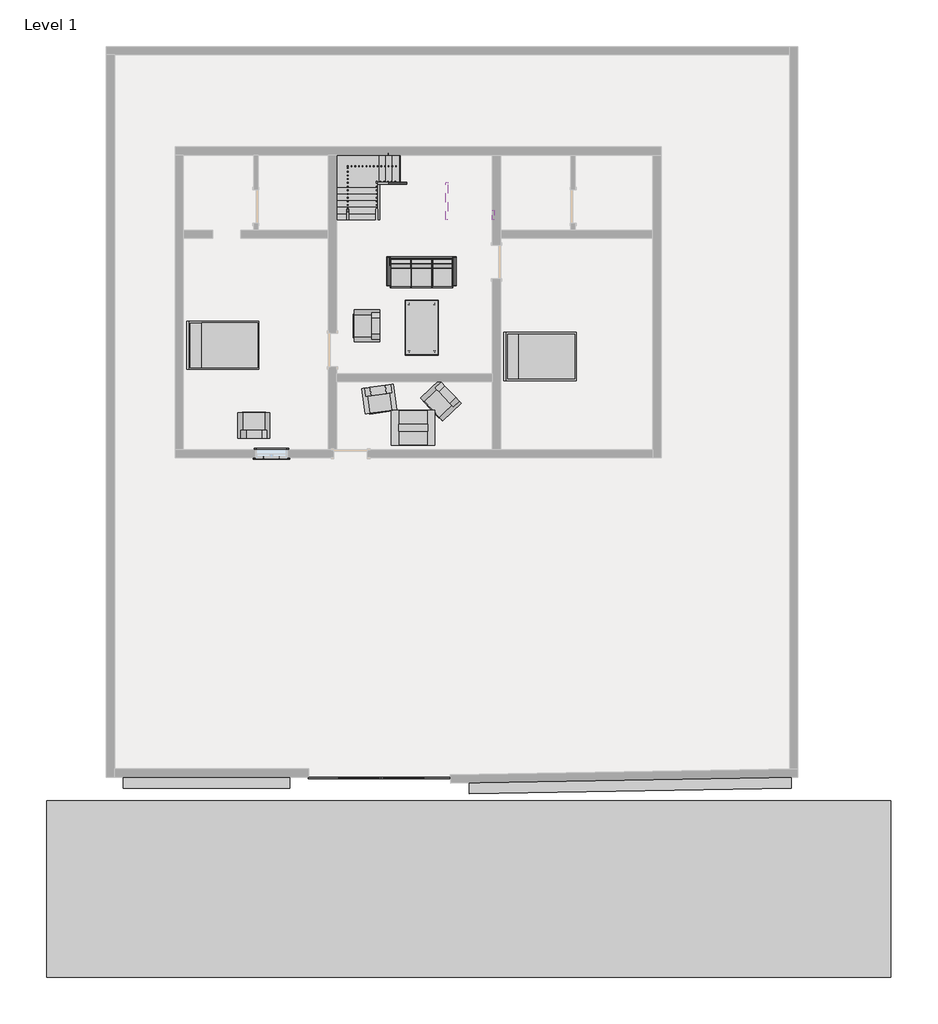
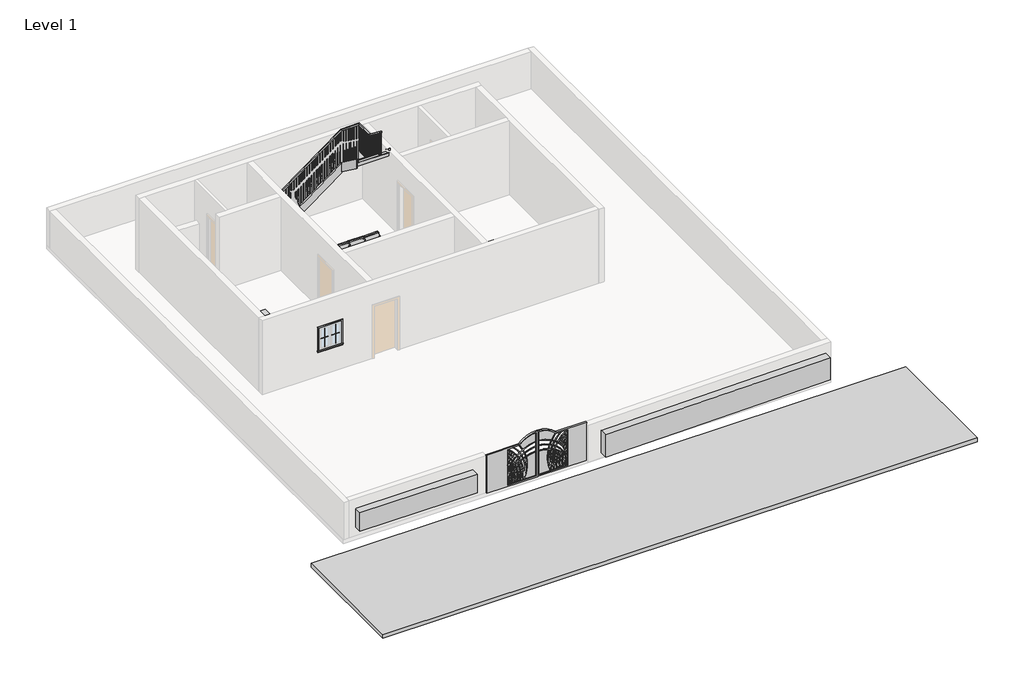
# One storey, part 2 of 2: 9 furniture elements, 8 proxies, 6 members, 1 railing, 1 stair flight.
"""IFC4 building model written with IfcOpenShell, lengths in millimetres."""

from ifc_helpers import new_model, si_unit, frame, origin, place, context, project, spatial, polyline, outline, extrude, faceted_brep, transform, mapped, element, save
from components import generic_models_1_generic_models_1_de819adb, generic_models_2_generic_models_2_5d5211df, generic_models_3_generic_models_3_fb8d8730, muntin_pattern_2x2_muntin_pattern_2x2_b3fe6957, muntin_pattern_2x2_muntin_pattern_2x2_3e0ecaf2, trim_window_exterior_flat_with_sill_41619996, trim_window_interior_flat_picture_frame_51c85655, gate_7956_gate_7956_2a423054, furniture_2fc85b74, furniture_29a9adb8, furniture_57072a26, bed_17739_bed_17739_15c61121, chair_lounge_11461_couch_0866092f, dining_table_14755_dining_table_14755_d89cb775, wood_and_glass_coffee_table_17065_wood_and_glass_coffee_dbc724b2, stair_flight_92e1e4df

model = new_model("IFC4")

# Units and contexts
model_context = context("Model", 3, world=origin())
ifc_project = project(units=[si_unit("LENGTHUNIT", "METRE", prefix="MILLI")], contexts=[model_context])

# Site, building, storey
site = spatial("IfcSite", under=ifc_project)
building = spatial("IfcBuilding", under=site)
storey = spatial("IfcBuildingStorey", under=building, Name="Level 1", Elevation=0.0)

# Proxies
placement = place(None, origin())
generic_models_1_generic_models_1_shape = generic_models_1_generic_models_1_de819adb(model_context)
element("IfcBuildingElementProxy", 1, Name="Generic Models 1 : Generic Models 1", ObjectType="Generic Models 1 : Generic Models 1", at=placement, inside=storey, context=model_context, shape_type="MappedRepresentation", body=[
    mapped(generic_models_1_generic_models_1_shape, transform((0.0, 0.0, 0.0), x_axis=(1.0, 0.0, 0.0), y_axis=(0.0, 1.0, 0.0), z_axis=(0.0, 0.0, 1.0))),
])
generic_models_2_generic_models_2_shape = generic_models_2_generic_models_2_5d5211df(model_context)
element("IfcBuildingElementProxy", 2, Name="Generic Models 2 : Generic Models 2", ObjectType="Generic Models 2 : Generic Models 2", at=placement, inside=storey, context=model_context, shape_type="MappedRepresentation", body=[
    mapped(generic_models_2_generic_models_2_shape, transform((0.0, 0.0, 0.0), x_axis=(1.0, 0.0, 0.0), y_axis=(0.0, 1.0, 0.0), z_axis=(0.0, 0.0, 1.0))),
])
generic_models_3_generic_models_3_shape = generic_models_3_generic_models_3_fb8d8730(model_context)
element("IfcBuildingElementProxy", 3, Name="Generic Models 3 : Generic Models 3", ObjectType="Generic Models 3 : Generic Models 3", at=placement, inside=storey, context=model_context, shape_type="MappedRepresentation", body=[
    mapped(generic_models_3_generic_models_3_shape, transform((0.0, 0.0, 0.0), x_axis=(1.0, 0.0, 0.0), y_axis=(0.0, 1.0, 0.0), z_axis=(0.0, 0.0, 1.0))),
])
muntin_pattern_2x2_muntin_pattern_2x2_shape = muntin_pattern_2x2_muntin_pattern_2x2_b3fe6957(model_context)
element("IfcBuildingElementProxy", 4, Name="Muntin Pattern_2x2 : Muntin Pattern_2x2", ObjectType="Muntin Pattern_2x2 : Muntin Pattern_2x2", at=placement, inside=storey, context=model_context, shape_type="MappedRepresentation", body=[
    mapped(muntin_pattern_2x2_muntin_pattern_2x2_shape, transform((-5069.3921642, -1799.3582394, 1136.9934313), x_axis=(-1.0, 0.0, 0.0), y_axis=(0.0, -1.0, 0.0), z_axis=(0.0, 0.0, 1.0))),
])
muntin_pattern_2x2_muntin_pattern_2x2_2_shape = muntin_pattern_2x2_muntin_pattern_2x2_3e0ecaf2(model_context)
element("IfcBuildingElementProxy", 5, Name="Muntin Pattern_2x2 : Muntin Pattern_2x2", ObjectType="Muntin Pattern_2x2 : Muntin Pattern_2x2", at=placement, inside=storey, context=model_context, shape_type="MappedRepresentation", body=[
    mapped(muntin_pattern_2x2_muntin_pattern_2x2_2_shape, transform((-5498.0171642, -1799.3582394, 1136.9934313), x_axis=(1.0, 0.0, 0.0), y_axis=(0.0, 1.0, 0.0), z_axis=(0.0, 0.0, 1.0))),
])
trim_window_exterior_flat_with_sill_shape = trim_window_exterior_flat_with_sill_41619996(model_context)
element("IfcBuildingElementProxy", 6, Name="Trim-Window-Exterior-Flat : with Sill", ObjectType="Trim-Window-Exterior-Flat : with Sill", at=placement, inside=storey, context=model_context, shape_type="MappedRepresentation", body=[
    mapped(trim_window_exterior_flat_with_sill_shape, transform((-5283.7046642, -1808.8832394, 1981.5434313), x_axis=(1.0, 0.0, 0.0), y_axis=(0.0, 0.0, 1.0), z_axis=(0.0, -1.0, 0.0))),
])
trim_window_interior_flat_picture_frame_shape = trim_window_interior_flat_picture_frame_51c85655(model_context)
element("IfcBuildingElementProxy", 7, Name="Trim-Window-Interior-Flat : Picture Frame", ObjectType="Trim-Window-Interior-Flat : Picture Frame", at=placement, inside=storey, context=model_context, shape_type="MappedRepresentation", body=[
    mapped(trim_window_interior_flat_picture_frame_shape, transform((-5283.7046642, -1580.2832394, 1981.5434313), x_axis=(-1.0, 0.0, 0.0), y_axis=(0.0, 0.0, 1.0), z_axis=(0.0, 1.0, 0.0))),
])
gate_7956_gate_7956_shape = gate_7956_gate_7956_2a423054(model_context)
element("IfcBuildingElementProxy", 8, Name="gate_7956 : gate_7956", ObjectType="gate_7956 : gate_7956", at=placement, inside=storey, context=model_context, shape_type="MappedRepresentation", body=[
    mapped(gate_7956_gate_7956_shape, transform((-2281.8126986, -10566.5980165, 0.0), x_axis=(1.0, 0.0, 0.0), y_axis=(0.0, 1.0, 0.0), z_axis=(0.0, 0.0, 1.0))),
])

# Furniture
furniture_shape = furniture_2fc85b74(model_context)
furniture_2_shape = furniture_29a9adb8(model_context)
furniture_3_shape = furniture_57072a26(model_context)
element("IfcFurniture", 9, at=placement, inside=storey, context=model_context, shape_type="MappedRepresentation", body=[
    mapped(furniture_shape, transform((-1166.392994, 2905.4688314, 0.0), x_axis=(1.0, 0.0, 0.0), y_axis=(0.0, 1.0, 0.0), z_axis=(0.0, 0.0, 1.0))),
    mapped(furniture_2_shape, transform((-1166.392994, 2905.4688314, 0.0), x_axis=(1.0, 0.0, 0.0), y_axis=(0.0, 1.0, 0.0), z_axis=(0.0, 0.0, 1.0))),
    mapped(furniture_3_shape, transform((-1166.392994, 2905.4688314, 0.0), x_axis=(1.0, 0.0, 0.0), y_axis=(0.0, 1.0, 0.0), z_axis=(0.0, 0.0, 1.0))),
])
bed_17739_bed_17739_shape = bed_17739_bed_17739_15c61121(model_context)
element("IfcFurniture", 10, ObjectType="Bed_17739 : Bed_17739", at=placement, inside=storey, context=model_context, shape_type="MappedRepresentation", body=[
    mapped(bed_17739_bed_17739_shape, transform((-6591.8046642, 1277.2167606, 0.0), x_axis=(0.0, 1.0, 0.0), y_axis=(-1.0, 0.0, 0.0), z_axis=(0.0, 0.0, 1.0))),
])
element("IfcFurniture", 11, ObjectType="Bed_17739 : Bed_17739", at=placement, inside=storey, context=model_context, shape_type="MappedRepresentation", body=[
    mapped(bed_17739_bed_17739_shape, transform((2107.6953358, 972.4167606, 0.0), x_axis=(0.0, 1.0, 0.0), y_axis=(-1.0, 0.0, 0.0), z_axis=(0.0, 0.0, 1.0))),
])
chair_lounge_11461_couch_shape = chair_lounge_11461_couch_0866092f(model_context)
element("IfcFurniture", 12, ObjectType="Chair-Lounge_11461 : Couch", at=placement, inside=storey, context=model_context, shape_type="MappedRepresentation", body=[
    mapped(chair_lounge_11461_couch_shape, transform((-5766.3046642, -1273.9095448, 0.0), x_axis=(-1.0, 0.0, 0.0), y_axis=(0.0, -1.0, 0.0), z_axis=(0.0, 0.0, 1.0))),
])
element("IfcFurniture", 13, ObjectType="Chair-Lounge_11461 : Couch", at=placement, inside=storey, context=model_context, shape_type="MappedRepresentation", body=[
    mapped(chair_lounge_11461_couch_shape, transform((-2311.9046642, 1810.6167606, 0.0), x_axis=(0.0, -1.0, 0.0), y_axis=(1.0, 0.0, 0.0), z_axis=(0.0, 0.0, 1.0))),
])
element("IfcFurniture", 14, ObjectType="Chair-Lounge_11461 : Couch", at=placement, inside=storey, context=model_context, shape_type="MappedRepresentation", body=[
    mapped(chair_lounge_11461_couch_shape, transform((-2372.9488995, 149.9169276, 0.0), x_axis=(0.9905324493396854, 0.1372787922627668, 0.0), y_axis=(-0.1372787922627668, 0.9905324493396854, 0.0), z_axis=(0.0, 0.0, 1.0))),
])
element("IfcFurniture", 15, ObjectType="Chair-Lounge_11461 : Couch", at=placement, inside=storey, context=model_context, shape_type="MappedRepresentation", body=[
    mapped(chair_lounge_11461_couch_shape, transform((-378.7925234, 1.7617886, 0.0), x_axis=(0.6894995564131368, -0.7242861048688479, 0.0), y_axis=(0.7242861048688479, 0.6894995564131368, 0.0), z_axis=(0.0, 0.0, 1.0))),
])
dining_table_14755_dining_table_14755_shape = dining_table_14755_dining_table_14755_d89cb775(model_context)
element("IfcFurniture", 16, ObjectType="Dining_table_14755 : Dining_table_14755", at=placement, inside=storey, context=model_context, shape_type="MappedRepresentation", body=[
    mapped(dining_table_14755_dining_table_14755_shape, transform((-711.7046642, 1010.5167606, 0.0), x_axis=(0.0, 1.0, 0.0), y_axis=(-1.0, 0.0, 0.0), z_axis=(0.0, 0.0, 1.0))),
])
wood_and_glass_coffee_table_17065_wood_and_glass_coffee_shape = wood_and_glass_coffee_table_17065_wood_and_glass_coffee_dbc724b2(model_context)
element("IfcFurniture", 17, ObjectType="Wood_and_Glass_Coffee_Table_17065 : Wood_and_Glass_Coffee_Table_17065", at=placement, inside=storey, context=model_context, shape_type="MappedRepresentation", body=[
    mapped(wood_and_glass_coffee_table_17065_wood_and_glass_coffee_shape, transform((-1397.5046642, -983.3832394, 0.0), x_axis=(1.0, 0.0, 0.0), y_axis=(0.0, 1.0, 0.0), z_axis=(0.0, 0.0, 1.0))),
])

# Members
element("IfcMember", 18, ObjectType="Stringer - 2\" Width", at=placement, inside=storey, context=model_context, shape_type="SweptSolid", body=[
    extrude(outline(polyline([(4718.9167606, 0.0), (4718.9167606, 147.6508226), (5113.281957, 147.6508226), (4911.6463024, 0.0), (4718.9167606, 0.0)])), frame((-3543.8046642, 0.0, 0.0), z_axis=(1.0, 0.0, 0.0), x_axis=(0.0, 1.0, 0.0)), (0.0, 0.0, 1.0), 50.8),
])
element("IfcMember", 19, ObjectType="Stringer - 2\" Width", at=placement, inside=storey, context=model_context, shape_type="SweptSolid", body=[
    extrude(outline(polyline([(1160.8387795, -1623.6098785), (1816.7484291, -743.5977653), (1816.7484291, -1253.6320422), (1160.8387795, -2133.6441554), (1160.8387795, -1623.6098785)])), frame((0.0, 6496.9167606, 0.0), z_axis=(0.0, 1.0, 0.0), x_axis=(0.0, 0.0, 1.0)), (0.0, 0.0, 1.0), 50.8),
])
element("IfcMember", 20, ObjectType="Stringer - 2\" Width", at=placement, inside=storey, context=model_context, shape_type="SweptSolid", body=[
    extrude(outline(polyline([(4718.9167606, 2948.0227901), (4718.9167606, 3141.9652405), (4979.1229954, 2948.0227901), (4718.9167606, 2948.0227901)])), frame((774.1953358, 0.0, 0.0), z_axis=(1.0, 0.0, 0.0), x_axis=(0.0, 1.0, 0.0)), (0.0, 0.0, 1.0), 50.8),
])
element("IfcMember", 21, ObjectType="Stringer - 2\" Width", at=placement, inside=storey, context=model_context, shape_type="SweptSolid", body=[
    extrude(outline(polyline([(4718.9167606, 0.0), (4718.9167606, 236.6522719), (5695.7536537, 951.9561753), (5695.7536537, 574.1747195), (4911.6463024, 0.0), (4718.9167606, 0.0)])), frame((-2368.6972892, 0.0, 0.0), z_axis=(1.0, 0.0, 0.0), x_axis=(0.0, 1.0, 0.0)), (0.0, 0.0, 1.0), 50.8),
])
element("IfcMember", 22, ObjectType="Stringer - 2\" Width", at=placement, inside=storey, context=model_context, shape_type="SweptSolid", body=[
    extrude(outline(polyline([(985.6438971, -2368.6972892), (611.3738041, -2368.6972892), (611.3738041, -2360.8087204), (2001.4389392, -495.8046642), (2376.0250342, -495.8046642), (2376.0250342, -503.2692636), (985.6438971, -2368.6972892)])), frame((0.0, 5695.7536537, 0.0), z_axis=(0.0, 1.0, 0.0), x_axis=(0.0, 0.0, 1.0)), (0.0, 0.0, 1.0), 50.8),
])
element("IfcMember", 23, ObjectType="Stringer - 2\" Width", at=placement, inside=storey, context=model_context, shape_type="SweptSolid", body=[
    extrude(outline(polyline([(5746.5536537, 2376.0250342), (5746.5536537, 2039.3022932), (5688.2891085, 2039.3022932), (4718.9167606, 2761.8155283), (4718.9167606, 3141.9652405), (5746.5536537, 2376.0250342)])), frame((-495.8046642, 0.0, 0.0), z_axis=(1.0, 0.0, 0.0), x_axis=(0.0, 1.0, 0.0)), (0.0, 0.0, 1.0), 50.8),
])

# Railing
element("IfcRailing", 24, ObjectType="Handrail - Rectangular", at=placement, inside=storey, context=model_context, shape_type="SolidModel", body=[
    faceted_brep([(-3213.6046642, 4718.9167606, 1046.9217391), (-3213.6046642, 4718.9167606, 983.5634439), (-3162.8046642, 4718.9167606, 983.5634439), (-3162.8046642, 4718.9167606, 1046.9217391), (-3213.6046642, 5555.0306195, 1670.112193), (-3213.6046642, 5571.8796657, 1619.312193), (-3162.8046642, 5571.8796657, 1619.312193), (-3162.8046642, 5555.0306195, 1670.112193), (-3213.6046642, 6217.5167606, 1670.112193), (-3213.6046642, 6217.5167606, 1619.312193), (-3162.8046642, 6166.7167606, 1619.312193), (-3162.8046642, 6166.7167606, 1670.112193), (-2551.1185231, 6217.5167606, 1670.112193), (-2534.269477, 6217.5167606, 1619.312193), (-2534.269477, 6166.7167606, 1619.312193), (-2551.1185231, 6166.7167606, 1670.112193), (-239.7185231, 6217.5167606, 3392.8948017), (-222.869477, 6217.5167606, 3342.0948017), (-222.869477, 6166.7167606, 3342.0948017), (-239.7185231, 6166.7167606, 3392.8948017), (494.7953358, 6217.5167606, 3392.8948017), (494.7953358, 6217.5167606, 3342.0948017), (443.9953358, 6166.7167606, 3342.0948017), (443.9953358, 6166.7167606, 3392.8948017), (494.7953358, 5483.0029017, 3392.8948017), (494.7953358, 5466.1538556, 3342.0948017), (443.9953358, 5466.1538556, 3342.0948017), (443.9953358, 5483.0029017, 3392.8948017), (494.7953358, 4718.9167606, 3962.4), (443.9953358, 4718.9167606, 3962.4), (443.9953358, 4718.9167606, 3899.0417047), (494.7953358, 4718.9167606, 3899.0417047)], [[[0, 1, 2, 3]], [[1, 0, 4, 5]], [[2, 1, 5, 6]], [[3, 2, 6, 7]], [[0, 3, 7, 4]], [[5, 4, 8, 9]], [[6, 5, 9, 10]], [[7, 6, 10, 11]], [[4, 7, 11, 8]], [[9, 8, 12, 13]], [[10, 9, 13, 14]], [[11, 10, 14, 15]], [[8, 11, 15, 12]], [[13, 12, 16, 17]], [[14, 13, 17, 18]], [[15, 14, 18, 19]], [[12, 15, 19, 16]], [[17, 16, 20, 21]], [[18, 17, 21, 22]], [[19, 18, 22, 23]], [[16, 19, 23, 20]], [[21, 20, 24, 25]], [[22, 21, 25, 26]], [[23, 22, 26, 27]], [[20, 23, 27, 24]], [[28, 29, 30, 31]], [[25, 24, 28, 31]], [[26, 25, 31, 30]], [[27, 26, 30, 29]], [[24, 27, 29, 28]]]),
    extrude(outline(polyline([(4779.2417606, 3854.0789718), (4779.2417606, 2915.4782609), (4760.1917606, 2915.4782609), (4760.1917606, 3868.2777296), (4779.2417606, 3854.0789718)])), frame((459.8703358, 0.0, 0.0), z_axis=(1.0, 0.0, 0.0), x_axis=(0.0, 1.0, 0.0)), (0.0, 0.0, 1.0), 19.05),
    extrude(outline(polyline([(4880.8417606, 3778.3522637), (4880.8417606, 2915.4782609), (4861.7917606, 2915.4782609), (4861.7917606, 3792.5510215), (4880.8417606, 3778.3522637)])), frame((459.8703358, 0.0, 0.0), z_axis=(1.0, 0.0, 0.0), x_axis=(0.0, 1.0, 0.0)), (0.0, 0.0, 1.0), 19.05),
    extrude(outline(polyline([(4982.4417606, 3702.6255557), (4982.4417606, 2782.9565217), (4963.3917606, 2782.9565217), (4963.3917606, 3716.8243134), (4982.4417606, 3702.6255557)])), frame((459.8703358, 0.0, 0.0), z_axis=(1.0, 0.0, 0.0), x_axis=(0.0, 1.0, 0.0)), (0.0, 0.0, 1.0), 19.05),
    extrude(outline(polyline([(5084.0417606, 3626.8988476), (5084.0417606, 2782.9565217), (5064.9917606, 2782.9565217), (5064.9917606, 3641.0976054), (5084.0417606, 3626.8988476)])), frame((459.8703358, 0.0, 0.0), z_axis=(1.0, 0.0, 0.0), x_axis=(0.0, 1.0, 0.0)), (0.0, 0.0, 1.0), 19.05),
    extrude(outline(polyline([(5185.6417606, 3551.1721395), (5185.6417606, 2650.4347826), (5166.5917606, 2650.4347826), (5166.5917606, 3565.3708973), (5185.6417606, 3551.1721395)])), frame((459.8703358, 0.0, 0.0), z_axis=(1.0, 0.0, 0.0), x_axis=(0.0, 1.0, 0.0)), (0.0, 0.0, 1.0), 19.05),
    extrude(outline(polyline([(5287.2417606, 3475.4454314), (5287.2417606, 2517.9130435), (5268.1917606, 2517.9130435), (5268.1917606, 3489.6441892), (5287.2417606, 3475.4454314)])), frame((459.8703358, 0.0, 0.0), z_axis=(1.0, 0.0, 0.0), x_axis=(0.0, 1.0, 0.0)), (0.0, 0.0, 1.0), 19.05),
    extrude(outline(polyline([(5388.8417606, 3399.7187234), (5388.8417606, 2517.9130435), (5369.7917606, 2517.9130435), (5369.7917606, 3413.9174811), (5388.8417606, 3399.7187234)])), frame((459.8703358, 0.0, 0.0), z_axis=(1.0, 0.0, 0.0), x_axis=(0.0, 1.0, 0.0)), (0.0, 0.0, 1.0), 19.05),
    extrude(outline(polyline([(5490.4417606, 3323.9920153), (5490.4417606, 2385.3913043), (5471.3917606, 2385.3913043), (5471.3917606, 3338.1907731), (5490.4417606, 3323.9920153)])), frame((459.8703358, 0.0, 0.0), z_axis=(1.0, 0.0, 0.0), x_axis=(0.0, 1.0, 0.0)), (0.0, 0.0, 1.0), 19.05),
    extrude(outline(polyline([(478.9203358, 5592.0417606), (478.9203358, 5572.9917606), (459.8703358, 5572.9917606), (459.8703358, 5592.0417606), (478.9203358, 5592.0417606)])), frame((0.0, 0.0, 2385.3913043), z_axis=(0.0, 0.0, 1.0), x_axis=(1.0, 0.0, 0.0)), (0.0, 0.0, 1.0), 956.7034973),
    extrude(outline(polyline([(478.9203358, 5693.6417606), (478.9203358, 5674.5917606), (459.8703358, 5674.5917606), (459.8703358, 5693.6417606), (478.9203358, 5693.6417606)])), frame((0.0, 0.0, 2252.8695652), z_axis=(0.0, 0.0, 1.0), x_axis=(1.0, 0.0, 0.0)), (0.0, 0.0, 1.0), 1089.2252364),
    extrude(outline(polyline([(478.9203358, 5795.2417606), (478.9203358, 5776.1917606), (459.8703358, 5776.1917606), (459.8703358, 5795.2417606), (478.9203358, 5795.2417606)])), frame((0.0, 0.0, 2252.8695652), z_axis=(0.0, 0.0, 1.0), x_axis=(1.0, 0.0, 0.0)), (0.0, 0.0, 1.0), 1089.2252364),
    extrude(outline(polyline([(478.9203358, 5896.8417606), (478.9203358, 5877.7917606), (459.8703358, 5877.7917606), (459.8703358, 5896.8417606), (478.9203358, 5896.8417606)])), frame((0.0, 0.0, 2252.8695652), z_axis=(0.0, 0.0, 1.0), x_axis=(1.0, 0.0, 0.0)), (0.0, 0.0, 1.0), 1089.2252364),
    extrude(outline(polyline([(478.9203358, 5998.4417606), (478.9203358, 5979.3917606), (459.8703358, 5979.3917606), (459.8703358, 5998.4417606), (478.9203358, 5998.4417606)])), frame((0.0, 0.0, 2252.8695652), z_axis=(0.0, 0.0, 1.0), x_axis=(1.0, 0.0, 0.0)), (0.0, 0.0, 1.0), 1089.2252364),
    extrude(outline(polyline([(478.9203358, 6100.0417606), (478.9203358, 6080.9917606), (459.8703358, 6080.9917606), (459.8703358, 6100.0417606), (478.9203358, 6100.0417606)])), frame((0.0, 0.0, 2252.8695652), z_axis=(0.0, 0.0, 1.0), x_axis=(1.0, 0.0, 0.0)), (0.0, 0.0, 1.0), 1089.2252364),
    extrude(outline(polyline([(358.2703358, 6201.6417606), (377.3203358, 6201.6417606), (377.3203358, 6182.5917606), (358.2703358, 6182.5917606), (358.2703358, 6201.6417606)])), frame((0.0, 0.0, 2252.8695652), z_axis=(0.0, 0.0, 1.0), x_axis=(1.0, 0.0, 0.0)), (0.0, 0.0, 1.0), 1089.2252364),
    extrude(outline(polyline([(256.6703358, 6201.6417606), (275.7203358, 6201.6417606), (275.7203358, 6182.5917606), (256.6703358, 6182.5917606), (256.6703358, 6201.6417606)])), frame((0.0, 0.0, 2252.8695652), z_axis=(0.0, 0.0, 1.0), x_axis=(1.0, 0.0, 0.0)), (0.0, 0.0, 1.0), 1089.2252364),
    extrude(outline(polyline([(155.0703358, 6201.6417606), (174.1203358, 6201.6417606), (174.1203358, 6182.5917606), (155.0703358, 6182.5917606), (155.0703358, 6201.6417606)])), frame((0.0, 0.0, 2252.8695652), z_axis=(0.0, 0.0, 1.0), x_axis=(1.0, 0.0, 0.0)), (0.0, 0.0, 1.0), 1089.2252364),
    extrude(outline(polyline([(53.4703358, 6201.6417606), (72.5203358, 6201.6417606), (72.5203358, 6182.5917606), (53.4703358, 6182.5917606), (53.4703358, 6201.6417606)])), frame((0.0, 0.0, 2252.8695652), z_axis=(0.0, 0.0, 1.0), x_axis=(1.0, 0.0, 0.0)), (0.0, 0.0, 1.0), 1089.2252364),
    extrude(outline(polyline([(-48.1296642, 6201.6417606), (-29.0796642, 6201.6417606), (-29.0796642, 6182.5917606), (-48.1296642, 6182.5917606), (-48.1296642, 6201.6417606)])), frame((0.0, 0.0, 2252.8695652), z_axis=(0.0, 0.0, 1.0), x_axis=(1.0, 0.0, 0.0)), (0.0, 0.0, 1.0), 1089.2252364),
    extrude(outline(polyline([(-149.7296642, 6201.6417606), (-130.6796642, 6201.6417606), (-130.6796642, 6182.5917606), (-149.7296642, 6182.5917606), (-149.7296642, 6201.6417606)])), frame((0.0, 0.0, 2252.8695652), z_axis=(0.0, 0.0, 1.0), x_axis=(1.0, 0.0, 0.0)), (0.0, 0.0, 1.0), 1089.2252364),
    extrude(outline(polyline([(3320.8822397, -251.3296642), (2252.8695652, -251.3296642), (2252.8695652, -232.2796642), (3335.0809975, -232.2796642), (3320.8822397, -251.3296642)])), frame((0.0, 6182.5917606, 0.0), z_axis=(0.0, 1.0, 0.0), x_axis=(0.0, 0.0, 1.0)), (0.0, 0.0, 1.0), 19.05),
    extrude(outline(polyline([(3245.1555316, -352.9296642), (2252.8695652, -352.9296642), (2252.8695652, -333.8796642), (3259.3542894, -333.8796642), (3245.1555316, -352.9296642)])), frame((0.0, 6182.5917606, 0.0), z_axis=(0.0, 1.0, 0.0), x_axis=(0.0, 0.0, 1.0)), (0.0, 0.0, 1.0), 19.05),
    extrude(outline(polyline([(3169.4288236, -454.5296642), (2252.8695652, -454.5296642), (2252.8695652, -435.4796642), (3183.6275813, -435.4796642), (3169.4288236, -454.5296642)])), frame((0.0, 6182.5917606, 0.0), z_axis=(0.0, 1.0, 0.0), x_axis=(0.0, 0.0, 1.0)), (0.0, 0.0, 1.0), 19.05),
    extrude(outline(polyline([(3093.7021155, -556.1296642), (2120.3478261, -556.1296642), (2120.3478261, -537.0796642), (3107.9008733, -537.0796642), (3093.7021155, -556.1296642)])), frame((0.0, 6182.5917606, 0.0), z_axis=(0.0, 1.0, 0.0), x_axis=(0.0, 0.0, 1.0)), (0.0, 0.0, 1.0), 19.05),
    extrude(outline(polyline([(3017.9754074, -657.7296642), (2120.3478261, -657.7296642), (2120.3478261, -638.6796642), (3032.1741652, -638.6796642), (3017.9754074, -657.7296642)])), frame((0.0, 6182.5917606, 0.0), z_axis=(0.0, 1.0, 0.0), x_axis=(0.0, 0.0, 1.0)), (0.0, 0.0, 1.0), 19.05),
    extrude(outline(polyline([(2942.2486993, -759.3296642), (1987.826087, -759.3296642), (1987.826087, -740.2796642), (2956.4474571, -740.2796642), (2942.2486993, -759.3296642)])), frame((0.0, 6182.5917606, 0.0), z_axis=(0.0, 1.0, 0.0), x_axis=(0.0, 0.0, 1.0)), (0.0, 0.0, 1.0), 19.05),
    extrude(outline(polyline([(2866.5219913, -860.9296642), (1987.826087, -860.9296642), (1987.826087, -841.8796642), (2880.720749, -841.8796642), (2866.5219913, -860.9296642)])), frame((0.0, 6182.5917606, 0.0), z_axis=(0.0, 1.0, 0.0), x_axis=(0.0, 0.0, 1.0)), (0.0, 0.0, 1.0), 19.05),
    extrude(outline(polyline([(2790.7952832, -962.5296642), (1855.3043478, -962.5296642), (1855.3043478, -943.4796642), (2804.994041, -943.4796642), (2790.7952832, -962.5296642)])), frame((0.0, 6182.5917606, 0.0), z_axis=(0.0, 1.0, 0.0), x_axis=(0.0, 0.0, 1.0)), (0.0, 0.0, 1.0), 19.05),
    extrude(outline(polyline([(2715.0685751, -1064.1296642), (1855.3043478, -1064.1296642), (1855.3043478, -1045.0796642), (2729.2673329, -1045.0796642), (2715.0685751, -1064.1296642)])), frame((0.0, 6182.5917606, 0.0), z_axis=(0.0, 1.0, 0.0), x_axis=(0.0, 0.0, 1.0)), (0.0, 0.0, 1.0), 19.05),
    extrude(outline(polyline([(2639.341867, -1165.7296642), (1722.7826087, -1165.7296642), (1722.7826087, -1146.6796642), (2653.5406248, -1146.6796642), (2639.341867, -1165.7296642)])), frame((0.0, 6182.5917606, 0.0), z_axis=(0.0, 1.0, 0.0), x_axis=(0.0, 0.0, 1.0)), (0.0, 0.0, 1.0), 19.05),
    extrude(outline(polyline([(2563.615159, -1267.3296642), (1590.2608696, -1267.3296642), (1590.2608696, -1248.2796642), (2577.8139167, -1248.2796642), (2563.615159, -1267.3296642)])), frame((0.0, 6182.5917606, 0.0), z_axis=(0.0, 1.0, 0.0), x_axis=(0.0, 0.0, 1.0)), (0.0, 0.0, 1.0), 19.05),
    extrude(outline(polyline([(2487.8884509, -1368.9296642), (1590.2608696, -1368.9296642), (1590.2608696, -1349.8796642), (2502.0872087, -1349.8796642), (2487.8884509, -1368.9296642)])), frame((0.0, 6182.5917606, 0.0), z_axis=(0.0, 1.0, 0.0), x_axis=(0.0, 0.0, 1.0)), (0.0, 0.0, 1.0), 19.05),
    extrude(outline(polyline([(2412.1617428, -1470.5296642), (1457.7391304, -1470.5296642), (1457.7391304, -1451.4796642), (2426.3605006, -1451.4796642), (2412.1617428, -1470.5296642)])), frame((0.0, 6182.5917606, 0.0), z_axis=(0.0, 1.0, 0.0), x_axis=(0.0, 0.0, 1.0)), (0.0, 0.0, 1.0), 19.05),
    extrude(outline(polyline([(2336.4350347, -1572.1296642), (1457.7391304, -1572.1296642), (1457.7391304, -1553.0796642), (2350.6337925, -1553.0796642), (2336.4350347, -1572.1296642)])), frame((0.0, 6182.5917606, 0.0), z_axis=(0.0, 1.0, 0.0), x_axis=(0.0, 0.0, 1.0)), (0.0, 0.0, 1.0), 19.05),
    extrude(outline(polyline([(2260.7083267, -1673.7296642), (1325.2173913, -1673.7296642), (1325.2173913, -1654.6796642), (2274.9070844, -1654.6796642), (2260.7083267, -1673.7296642)])), frame((0.0, 6182.5917606, 0.0), z_axis=(0.0, 1.0, 0.0), x_axis=(0.0, 0.0, 1.0)), (0.0, 0.0, 1.0), 19.05),
    extrude(outline(polyline([(2184.9816186, -1775.3296642), (1325.2173913, -1775.3296642), (1325.2173913, -1756.2796642), (2199.1803764, -1756.2796642), (2184.9816186, -1775.3296642)])), frame((0.0, 6182.5917606, 0.0), z_axis=(0.0, 1.0, 0.0), x_axis=(0.0, 0.0, 1.0)), (0.0, 0.0, 1.0), 19.05),
    extrude(outline(polyline([(2109.2549105, -1876.9296642), (1192.6956522, -1876.9296642), (1192.6956522, -1857.8796642), (2123.4536683, -1857.8796642), (2109.2549105, -1876.9296642)])), frame((0.0, 6182.5917606, 0.0), z_axis=(0.0, 1.0, 0.0), x_axis=(0.0, 0.0, 1.0)), (0.0, 0.0, 1.0), 19.05),
    extrude(outline(polyline([(2033.5282025, -1978.5296642), (1060.173913, -1978.5296642), (1060.173913, -1959.4796642), (2047.7269602, -1959.4796642), (2033.5282025, -1978.5296642)])), frame((0.0, 6182.5917606, 0.0), z_axis=(0.0, 1.0, 0.0), x_axis=(0.0, 0.0, 1.0)), (0.0, 0.0, 1.0), 19.05),
    extrude(outline(polyline([(1957.8014944, -2080.1296642), (1060.173913, -2080.1296642), (1060.173913, -2061.0796642), (1972.0002521, -2061.0796642), (1957.8014944, -2080.1296642)])), frame((0.0, 6182.5917606, 0.0), z_axis=(0.0, 1.0, 0.0), x_axis=(0.0, 0.0, 1.0)), (0.0, 0.0, 1.0), 19.05),
    extrude(outline(polyline([(1882.0747863, -2181.7296642), (927.6521739, -2181.7296642), (927.6521739, -2162.6796642), (1896.2735441, -2162.6796642), (1882.0747863, -2181.7296642)])), frame((0.0, 6182.5917606, 0.0), z_axis=(0.0, 1.0, 0.0), x_axis=(0.0, 0.0, 1.0)), (0.0, 0.0, 1.0), 19.05),
    extrude(outline(polyline([(1806.3480782, -2283.3296642), (927.6521739, -2283.3296642), (927.6521739, -2264.2796642), (1820.546836, -2264.2796642), (1806.3480782, -2283.3296642)])), frame((0.0, 6182.5917606, 0.0), z_axis=(0.0, 1.0, 0.0), x_axis=(0.0, 0.0, 1.0)), (0.0, 0.0, 1.0), 19.05),
    extrude(outline(polyline([(1730.6213702, -2384.9296642), (795.1304348, -2384.9296642), (795.1304348, -2365.8796642), (1744.8201279, -2365.8796642), (1730.6213702, -2384.9296642)])), frame((0.0, 6182.5917606, 0.0), z_axis=(0.0, 1.0, 0.0), x_axis=(0.0, 0.0, 1.0)), (0.0, 0.0, 1.0), 19.05),
    extrude(outline(polyline([(1654.8946621, -2486.5296642), (795.1304348, -2486.5296642), (795.1304348, -2467.4796642), (1669.0934198, -2467.4796642), (1654.8946621, -2486.5296642)])), frame((0.0, 6182.5917606, 0.0), z_axis=(0.0, 1.0, 0.0), x_axis=(0.0, 0.0, 1.0)), (0.0, 0.0, 1.0), 19.05),
    extrude(outline(polyline([(-2588.1296642, 6201.6417606), (-2569.0796642, 6201.6417606), (-2569.0796642, 6182.5917606), (-2588.1296642, 6182.5917606), (-2588.1296642, 6201.6417606)])), frame((0.0, 0.0, 795.1304348), z_axis=(0.0, 0.0, 1.0), x_axis=(1.0, 0.0, 0.0)), (0.0, 0.0, 1.0), 824.1817582),
    extrude(outline(polyline([(-2689.7296642, 6201.6417606), (-2670.6796642, 6201.6417606), (-2670.6796642, 6182.5917606), (-2689.7296642, 6182.5917606), (-2689.7296642, 6201.6417606)])), frame((0.0, 0.0, 795.1304348), z_axis=(0.0, 0.0, 1.0), x_axis=(1.0, 0.0, 0.0)), (0.0, 0.0, 1.0), 824.1817582),
    extrude(outline(polyline([(-2791.3296642, 6201.6417606), (-2772.2796642, 6201.6417606), (-2772.2796642, 6182.5917606), (-2791.3296642, 6182.5917606), (-2791.3296642, 6201.6417606)])), frame((0.0, 0.0, 795.1304348), z_axis=(0.0, 0.0, 1.0), x_axis=(1.0, 0.0, 0.0)), (0.0, 0.0, 1.0), 824.1817582),
    extrude(outline(polyline([(-2892.9296642, 6201.6417606), (-2873.8796642, 6201.6417606), (-2873.8796642, 6182.5917606), (-2892.9296642, 6182.5917606), (-2892.9296642, 6201.6417606)])), frame((0.0, 0.0, 795.1304348), z_axis=(0.0, 0.0, 1.0), x_axis=(1.0, 0.0, 0.0)), (0.0, 0.0, 1.0), 824.1817582),
    extrude(outline(polyline([(-2994.5296642, 6201.6417606), (-2975.4796642, 6201.6417606), (-2975.4796642, 6182.5917606), (-2994.5296642, 6182.5917606), (-2994.5296642, 6201.6417606)])), frame((0.0, 0.0, 795.1304348), z_axis=(0.0, 0.0, 1.0), x_axis=(1.0, 0.0, 0.0)), (0.0, 0.0, 1.0), 824.1817582),
    extrude(outline(polyline([(-3096.1296642, 6201.6417606), (-3077.0796642, 6201.6417606), (-3077.0796642, 6182.5917606), (-3096.1296642, 6182.5917606), (-3096.1296642, 6201.6417606)])), frame((0.0, 0.0, 795.1304348), z_axis=(0.0, 0.0, 1.0), x_axis=(1.0, 0.0, 0.0)), (0.0, 0.0, 1.0), 824.1817582),
    extrude(outline(polyline([(-3197.7296642, 6131.7917606), (-3197.7296642, 6150.8417606), (-3178.6796642, 6150.8417606), (-3178.6796642, 6131.7917606), (-3197.7296642, 6131.7917606)])), frame((0.0, 0.0, 795.1304348), z_axis=(0.0, 0.0, 1.0), x_axis=(1.0, 0.0, 0.0)), (0.0, 0.0, 1.0), 824.1817582),
    extrude(outline(polyline([(-3197.7296642, 6030.1917606), (-3197.7296642, 6049.2417606), (-3178.6796642, 6049.2417606), (-3178.6796642, 6030.1917606), (-3197.7296642, 6030.1917606)])), frame((0.0, 0.0, 795.1304348), z_axis=(0.0, 0.0, 1.0), x_axis=(1.0, 0.0, 0.0)), (0.0, 0.0, 1.0), 824.1817582),
    extrude(outline(polyline([(-3197.7296642, 5928.5917606), (-3197.7296642, 5947.6417606), (-3178.6796642, 5947.6417606), (-3178.6796642, 5928.5917606), (-3197.7296642, 5928.5917606)])), frame((0.0, 0.0, 795.1304348), z_axis=(0.0, 0.0, 1.0), x_axis=(1.0, 0.0, 0.0)), (0.0, 0.0, 1.0), 824.1817582),
    extrude(outline(polyline([(-3197.7296642, 5826.9917606), (-3197.7296642, 5846.0417606), (-3178.6796642, 5846.0417606), (-3178.6796642, 5826.9917606), (-3197.7296642, 5826.9917606)])), frame((0.0, 0.0, 795.1304348), z_axis=(0.0, 0.0, 1.0), x_axis=(1.0, 0.0, 0.0)), (0.0, 0.0, 1.0), 824.1817582),
    extrude(outline(polyline([(-3197.7296642, 5725.3917606), (-3197.7296642, 5744.4417606), (-3178.6796642, 5744.4417606), (-3178.6796642, 5725.3917606), (-3197.7296642, 5725.3917606)])), frame((0.0, 0.0, 795.1304348), z_axis=(0.0, 0.0, 1.0), x_axis=(1.0, 0.0, 0.0)), (0.0, 0.0, 1.0), 824.1817582),
    extrude(outline(polyline([(-3197.7296642, 5623.7917606), (-3197.7296642, 5642.8417606), (-3178.6796642, 5642.8417606), (-3178.6796642, 5623.7917606), (-3197.7296642, 5623.7917606)])), frame((0.0, 0.0, 795.1304348), z_axis=(0.0, 0.0, 1.0), x_axis=(1.0, 0.0, 0.0)), (0.0, 0.0, 1.0), 824.1817582),
    extrude(outline(polyline([(5541.2417606, 1596.4764873), (5541.2417606, 662.6086957), (5522.1917606, 662.6086957), (5522.1917606, 1582.2777296), (5541.2417606, 1596.4764873)])), frame((-3197.7296642, 0.0, 0.0), z_axis=(1.0, 0.0, 0.0), x_axis=(0.0, 1.0, 0.0)), (0.0, 0.0, 1.0), 19.05),
    extrude(outline(polyline([(5439.6417606, 1520.7497793), (5439.6417606, 662.6086957), (5420.5917606, 662.6086957), (5420.5917606, 1506.5510215), (5439.6417606, 1520.7497793)])), frame((-3197.7296642, 0.0, 0.0), z_axis=(1.0, 0.0, 0.0), x_axis=(0.0, 1.0, 0.0)), (0.0, 0.0, 1.0), 19.05),
    extrude(outline(polyline([(5338.0417606, 1445.0230712), (5338.0417606, 530.0869565), (5318.9917606, 530.0869565), (5318.9917606, 1430.8243134), (5338.0417606, 1445.0230712)])), frame((-3197.7296642, 0.0, 0.0), z_axis=(1.0, 0.0, 0.0), x_axis=(0.0, 1.0, 0.0)), (0.0, 0.0, 1.0), 19.05),
    extrude(outline(polyline([(5236.4417606, 1369.2963631), (5236.4417606, 397.5652174), (5217.3917606, 397.5652174), (5217.3917606, 1355.0976054), (5236.4417606, 1369.2963631)])), frame((-3197.7296642, 0.0, 0.0), z_axis=(1.0, 0.0, 0.0), x_axis=(0.0, 1.0, 0.0)), (0.0, 0.0, 1.0), 19.05),
    extrude(outline(polyline([(5134.8417606, 1293.569655), (5134.8417606, 397.5652174), (5115.7917606, 397.5652174), (5115.7917606, 1279.3708973), (5134.8417606, 1293.569655)])), frame((-3197.7296642, 0.0, 0.0), z_axis=(1.0, 0.0, 0.0), x_axis=(0.0, 1.0, 0.0)), (0.0, 0.0, 1.0), 19.05),
    extrude(outline(polyline([(5033.2417606, 1217.842947), (5033.2417606, 265.0434783), (5014.1917606, 265.0434783), (5014.1917606, 1203.6441892), (5033.2417606, 1217.842947)])), frame((-3197.7296642, 0.0, 0.0), z_axis=(1.0, 0.0, 0.0), x_axis=(0.0, 1.0, 0.0)), (0.0, 0.0, 1.0), 19.05),
    extrude(outline(polyline([(4931.6417606, 1142.1162389), (4931.6417606, 265.0434783), (4912.5917606, 265.0434783), (4912.5917606, 1127.9174811), (4931.6417606, 1142.1162389)])), frame((-3197.7296642, 0.0, 0.0), z_axis=(1.0, 0.0, 0.0), x_axis=(0.0, 1.0, 0.0)), (0.0, 0.0, 1.0), 19.05),
    extrude(outline(polyline([(4830.0417606, 1066.3895308), (4830.0417606, 132.5217391), (4810.9917606, 132.5217391), (4810.9917606, 1052.1907731), (4830.0417606, 1066.3895308)])), frame((-3197.7296642, 0.0, 0.0), z_axis=(1.0, 0.0, 0.0), x_axis=(0.0, 1.0, 0.0)), (0.0, 0.0, 1.0), 19.05),
    extrude(outline(polyline([(459.8703358, 6201.6417606), (478.9203358, 6201.6417606), (478.9203358, 6182.5917606), (459.8703358, 6182.5917606), (459.8703358, 6201.6417606)])), frame((0.0, 0.0, 2252.8695652), z_axis=(0.0, 0.0, 1.0), x_axis=(1.0, 0.0, 0.0)), (0.0, 0.0, 1.0), 1089.2252364),
    extrude(outline(polyline([(-3197.7296642, 6182.5917606), (-3197.7296642, 6201.6417606), (-3178.6796642, 6201.6417606), (-3178.6796642, 6182.5917606), (-3197.7296642, 6182.5917606)])), frame((0.0, 0.0, 795.1304348), z_axis=(0.0, 0.0, 1.0), x_axis=(1.0, 0.0, 0.0)), (0.0, 0.0, 1.0), 824.1817582),
    extrude(outline(polyline([(4737.9667606, 3884.842947), (4737.9667606, 2915.4782609), (4718.9167606, 2915.4782609), (4718.9167606, 3899.0417047), (4737.9667606, 3884.842947)])), frame((459.8703358, 0.0, 0.0), z_axis=(1.0, 0.0, 0.0), x_axis=(0.0, 1.0, 0.0)), (0.0, 0.0, 1.0), 19.05),
    extrude(outline(polyline([(4737.9667606, 997.7622016), (4737.9667606, 132.5217391), (4718.9167606, 132.5217391), (4718.9167606, 983.5634439), (4737.9667606, 997.7622016)])), frame((-3197.7296642, 0.0, 0.0), z_axis=(1.0, 0.0, 0.0), x_axis=(0.0, 1.0, 0.0)), (0.0, 0.0, 1.0), 19.05),
])

# Stair flight
stair_flight_shape = stair_flight_92e1e4df(model_context)
element("IfcStairFlight", 25, ObjectType="2\" Tread 1\" Nosing 1/4\" Riser", at=placement, inside=storey, context=model_context, shape_type="MappedRepresentation", body=[
    mapped(stair_flight_shape, transform((0.0, 0.0, 0.0), x_axis=(1.0, 0.0, 0.0), y_axis=(0.0, 1.0, 0.0), z_axis=(0.0, 0.0, 1.0))),
])

save(model, "model.ifc")

# Revit data of these elements
# Type "Muntin Pattern_2x2 : Muntin Pattern_2x2"
#   Width [instance default] = 4' - 0"
#   Thickness = 0' - 0 1/2"
#   Height [instance default] = 4' - 0"
#   Distance = 0' - 0 3/4"
#   Interior Material [instance default] = none
#   Exterior Material [instance default] = none
#   Default Elevation = 0
# Type "Trim-Window-Exterior-Flat : with Sill"
#   Trim Width = 0' - 2 1/4"
#   Trim Thickness_Picture Frame = 0' - 1 1/4"
#   Trim Thickness_with Sill = 0' - 0 3/4"
#   Sill Thickness = 0' - 1 1/4"
#   Opening Width [instance default] = 2' - 0"
#   Opening Height [instance default] = 3' - 0"
#   Default Elevation = 4' - 0"
#   Sill = yes
#   Picture Frame = no
#   Trim Material [instance default] = none
# Type "Trim-Window-Interior-Flat : Picture Frame"
#   Trim Thickness_Picture Frame = 0' - 1 1/4"
#   Trim Width = 0' - 2 1/4"
#   Trim Thickness_with Sill = 0' - 0 3/4"
#   Sill Thickness = 0' - 1 1/4"
#   Opening Width [instance default] = 2' - 0"
#   Opening Height [instance default] = 3' - 0"
#   Default Elevation = 4' - 0"
#   Sill = no
#   Picture Frame = yes
#   Trim Material [instance default] = none
# Type "gate_7956 : gate_7956"
#   m.s. sheet = none
#   2" x2" pipe = none
#   1"x1"pipe = none
#   Default Elevation = 0
# Type
#   Width [instance] = 6' - 3.19685"
#   Default Elevation = 0
# Type "Bed_17739 : Bed_17739"
#   Default Elevation = 0
# Type "Chair-Lounge_11461 : Couch"
#   Default Elevation = 0
#   Assembly Code = ""
# Type "Dining_table_14755 : Dining_table_14755"
#   Lengte [instance default] = 4' - 11.05512"
#   Breedte [instance default] = 2' - 11.43307"
#   Tafelblad = none
#   Poten = none
#   Default Elevation = 0
# Type "Wood_and_Glass_Coffee_Table_17065 : Wood_and_Glass_Coffee_Table_17065"
#   Coffee Table Wood Width = 0' - 7.87402"
#   Coffee Table Width = 3' - 2.17592"
#   Coffee Table Length = 3' - 11.24409"
#   Wood and Glass Coffee Table - Wood = Wood and Glass Coffee Table - Wood
#   Wood and Glass Coffee Table - Glass = Wood and Glass Coffee Table - Glass
#   Default Elevation = 0
# Type "Handrail - Rectangular"
#   Assembly Code = "C2010400"
#   built-in parameter 1008612 = 0.0416667 (stored number, unit not read)
#   built-in parameter 1008611 = 0.0416667 (stored number, unit not read)
#   built-in parameter 1008609 = 0.333333 (stored number, unit not read)
#   built-in parameter 1008604 = 0.166667 (stored number, unit not read)
#   built-in parameter 1008603 = 0.166667 (stored number, unit not read)
#   Railing Height = 3' - 0"
#   built-in parameter 1008630 = 2
#   built-in parameter 1008610 = 2
#   built-in parameter 1008618 = Baluster - Square : 3/4"
# Element 1 (IfcBuildingElementProxy, "Generic Models 1 : Generic Models 1")
#   Phase Created = New Construction
# Element 2 (IfcBuildingElementProxy, "Generic Models 2 : Generic Models 2")
#   Phase Created = New Construction
#   Materials on its faces: "Parking Stripe"
# Element 3 (IfcBuildingElementProxy, "Generic Models 3 : Generic Models 3")
#   Phase Created = New Construction
#   Materials on its faces: "Parking Stripe"
# Elements 4, 5 (IfcBuildingElementProxy, "Muntin Pattern_2x2 : Muntin Pattern_2x2")
#   Width = 0' - 11 5/8"
#   Height = 2' - 6 1/2"
#   Interior Material = Wood - Stained
#   Exterior Material = Clad - White
#   Phase Created = New Construction
#   Materials on its faces: "Clad - White", "Wood - Stained"
# Element 6 (IfcBuildingElementProxy, "Trim-Window-Exterior-Flat : with Sill")
#   Opening Width = 2' - 10"
#   Opening Height = 3' - 0"
#   Trim Material = Clad - White
#   Phase Created = New Construction
#   Materials on its faces: "Clad - White"
# Element 7 (IfcBuildingElementProxy, "Trim-Window-Interior-Flat : Picture Frame")
#   Opening Width = 2' - 10"
#   Opening Height = 3' - 0"
#   Trim Material = Wood - Stained
#   Phase Created = New Construction
#   Materials on its faces: "Wood - Stained"
# Element 8 (IfcBuildingElementProxy, "gate_7956 : gate_7956")
#   Phase Created = New Construction
# Element 9 (IfcFurniture)
#   Width = 6' - 3.19685"
#   Phase Created = New Construction
# Elements 10, 11 (IfcFurniture, "Bed_17739 : Bed_17739")
#   Phase Created = New Construction
#   Materials on its faces: "legs", "sheets", "bed frame", "Blanket"
# Elements 12, 13, 14, 15 (IfcFurniture, "Chair-Lounge_11461 : Couch")
#   Phase Created = New Construction
# Element 16 (IfcFurniture, "Dining_table_14755 : Dining_table_14755")
#   Lengte = 4' - 11.05512"
#   Breedte = 2' - 11.43307"
#   Phase Created = New Construction
# Element 17 (IfcFurniture, "Wood_and_Glass_Coffee_Table_17065 : Wood_and_Glass_Coffee_Table_17065")
#   Phase Created = New Construction
#   Materials on its faces: "Wood and Glass Coffee Table - Wood", "Wood and Glass Coffee Table - Glass"
# Elements 18, 19, 20, 21, 22, 23 (IfcMember, "Stringer - 2\" Width")
#   Phase Created = New Construction
# Element 24 (IfcRailing, "Handrail - Rectangular")
#   Phase Created = New Construction
# Element 25 (IfcStairFlight, "2\" Tread 1\" Nosing 1/4\" Riser")
#   Phase Created = New Construction
# Materials
#   "Wood and Glass Coffee Table - Wood": class "Generic", colour RGB 120 120 120, transparency 0, Cost = 0
#   "Wood and Glass Coffee Table - Glass": class "Generic", colour RGB 120 120 120, transparency 0, Cost = 0
#   "Parking Stripe": class "Paint", colour RGB 250 250 91, transparency 0, Cost = 0
#   "Clad - White": class "Wood", colour RGB 242 242 238, transparency 0, Cost = 0
#   "Wood - Stained": class "Wood", colour RGB 224 178 126, transparency 0, Cost = 0
#   "legs": colour RGB 90 73 37, transparency 0, Cost = 0
#   "sheets": colour RGB 200 195 176, transparency 0, Cost = 0
#   "bed frame": colour RGB 90 73 37, transparency 0, Cost = 0
#   "Blanket": class "System", colour RGB 59 0 1, transparency 0, Cost = 0
